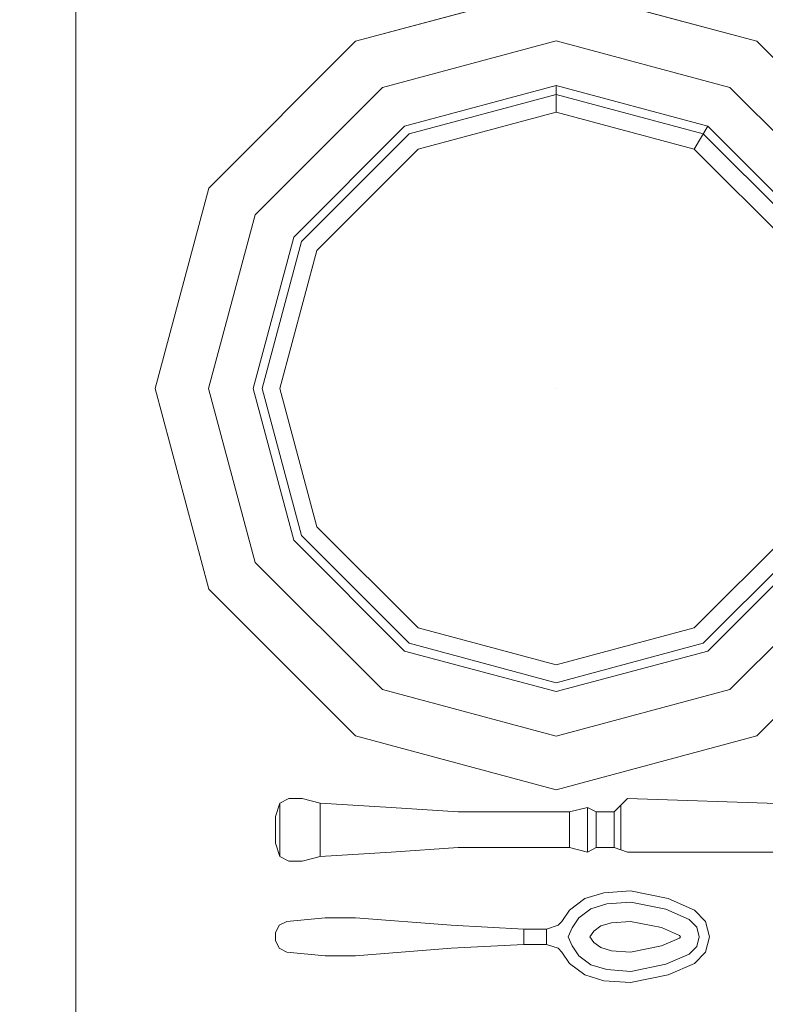
# Model space of a CAD drawing. Units: inches. Extents: x 375 to 1122, y 27 to 1069.
# Tile 116 of 155: x 705.14 to 715.44, y 886.61 to 900.21. Entities that reach past the tile are written whole.
import ezdxf

# ---------------------------------------------------------------- set-up
doc = ezdxf.new("R2010")
doc.units = ezdxf.units.IN
doc.layers.add('A-ANNO-DIMS', color=2, linetype='Continuous', lineweight=18)
doc.layers.add('Furniture', color=30, linetype='Continuous', lineweight=18)
doc.styles.get("Standard").update_dxf_attribs({"font": 'arial.ttf'})
doc.dimstyles.new('ISO-25', dxfattribs={"dimtxt": 12, "dimasz": 2.5, "dimexe": 1.5, "dimexo": 1.5, "dimtad": 1, "dimdec": 1, "dimlunit": 3, "dimtxsty": 'Standard', "dimblk": 'ARCHTICK', "dimcen": 2.5, "dimadec": 0, "dimazin": 0, "dimtfac": 1, "dimtdec": 1, "dimtmove": 0, "dimatfit": 3, "dimfxl": 1.5, "dimfxlon": 1, "dimarcsym": 0})

# ---------------------------------------------------------------- blocks, each defined once
blk = doc.blocks.new('A$C403C54AD')
blk.add_line((0.83575, 0.52421, -0.0006), (1.99923, 0.52421, -0.0006))
at = {"linetype": 'ByBlock'}
for points, invisible_edges in [([(1.01094, 0.81008, -0.00874), (1.02018, 0.79408, -0.00874), (0.97623, 0.75014, -0.00874), (0.96024, 0.75938, -0.00874)], 5), ([(1.02787, 0.78075, -0.02259), (1.01094, 0.81008, -0.01335), (0.96024, 0.75938, -0.01335), (0.98956, 0.74244, -0.02259)], 5), ([(1.17085, 0.74244, -0.02259), (1.20017, 0.75938, -0.01335), (1.14947, 0.81008, -0.01335), (1.13254, 0.78075, -0.02259)], 5), ([(1.20017, 0.75938, -0.00874), (1.18418, 0.75014, -0.00874), (1.14023, 0.79408, -0.00874), (1.14947, 0.81008, -0.00874)], 5), ([(1.02018, 0.79408, -0.00874), (1.02941, 0.77809, -0.01489), (0.99223, 0.74091, -0.01489), (0.97623, 0.75014, -0.00874)], 5), ([(1.18418, 0.75014, -0.00874), (1.16818, 0.74091, -0.01489), (1.131, 0.77809, -0.01489), (1.14023, 0.79408, -0.00874)], 5), ([(1.0802, 0.7917, -0.01489), (1.0802, 0.69011, -0.01489), (1.0802, 0.69011, -0.01489), (1.02941, 0.77809, -0.01489)], 5), ([(1.131, 0.77809, -0.01489), (1.0802, 0.69011, -0.01489), (1.0802, 0.69011, -0.01489), (1.0802, 0.7917, -0.01489)], 5), ([(1.03249, 0.77276, -0.03183), (1.02787, 0.78075, -0.02259), (0.98956, 0.74244, -0.02259), (0.99756, 0.73783, -0.03183)], 1), ([(1.16285, 0.73783, -0.03183), (1.17085, 0.74244, -0.02259), (1.13254, 0.78075, -0.02259), (1.12792, 0.77276, -0.03183)], 5), ([(1.02941, 0.77809, -0.01489), (1.0802, 0.69011, -0.01489), (1.0802, 0.69011, -0.01489), (0.99223, 0.74091, -0.01489)], 5), ([(1.16818, 0.74091, -0.01489), (1.0802, 0.69011, -0.01489), (1.0802, 0.69011, -0.01489), (1.131, 0.77809, -0.01489)], 5), ([(0.96024, 0.75938, -0.00874), (0.97623, 0.75014, -0.00874), (0.96015, 0.69011, -0.00874), (0.94168, 0.69011, -0.00874)], 5), ([(0.98956, 0.74244, -0.02259), (0.96024, 0.75938, -0.01335), (0.94168, 0.69011, -0.01335), (0.97554, 0.69011, -0.02259)], 5), ([(1.18487, 0.69011, -0.02259), (1.21873, 0.69011, -0.01335), (1.20017, 0.75938, -0.01335), (1.17085, 0.74244, -0.02259)], 5), ([(1.21873, 0.69011, -0.00874), (1.20026, 0.69011, -0.00874), (1.18418, 0.75014, -0.00874), (1.20017, 0.75938, -0.00874)], 5), ([(0.97623, 0.75014, -0.00874), (0.99223, 0.74091, -0.01489), (0.97862, 0.69011, -0.01489), (0.96015, 0.69011, -0.00874)], 5), ([(1.20026, 0.69011, -0.00874), (1.18179, 0.69011, -0.01489), (1.16818, 0.74091, -0.01489), (1.18418, 0.75014, -0.00874)], 5), ([(1.17563, 0.69011, -0.03183), (1.18487, 0.69011, -0.02259), (1.17085, 0.74244, -0.02259), (1.16285, 0.73783, -0.03183)], 5), ([(0.99223, 0.74091, -0.01489), (1.0802, 0.69011, -0.01489), (1.0802, 0.69011, -0.01489), (0.97862, 0.69011, -0.01489)], 5), ([(1.18179, 0.69011, -0.01489), (1.0802, 0.69011, -0.01489), (1.0802, 0.69011, -0.01489), (1.16818, 0.74091, -0.01489)], 5), ([(0.94168, 0.69011, -0.00874), (0.96015, 0.69011, -0.00874), (0.97623, 0.63008, -0.00874), (0.96024, 0.62085, -0.00874)], 5), ([(0.97554, 0.69011, -0.02259), (0.94168, 0.69011, -0.01335), (0.96024, 0.62085, -0.01335), (0.98956, 0.63778, -0.02259)], 5), ([(0.96015, 0.69011, -0.00874), (0.97862, 0.69011, -0.01489), (0.99223, 0.63932, -0.01489), (0.97623, 0.63008, -0.00874)], 5), ([(0.98477, 0.69011, -0.03183), (0.97554, 0.69011, -0.02259), (0.98956, 0.63778, -0.02259), (0.99756, 0.6424, -0.03183)], 4), ([(0.97862, 0.69011, -0.01489), (1.0802, 0.69011, -0.01489), (1.0802, 0.69011, -0.01489), (0.99223, 0.63932, -0.01489)], 5), ([(0.99223, 0.63932, -0.01489), (1.0802, 0.69011, -0.01489), (1.0802, 0.69011, -0.01489), (1.02941, 0.60214, -0.01489)], 5), ([(1.02941, 0.60214, -0.01489), (1.0802, 0.69011, -0.01489), (1.0802, 0.69011, -0.01489), (1.0802, 0.58853, -0.01489)], 5), ([(1.0802, 0.58853, -0.01489), (1.0802, 0.69011, -0.01489), (1.0802, 0.69011, -0.01489), (1.131, 0.60214, -0.01489)], 5), ([(1.131, 0.60214, -0.01489), (1.0802, 0.69011, -0.01489), (1.0802, 0.69011, -0.01489), (1.16818, 0.63932, -0.01489)], 5), ([(1.16818, 0.63932, -0.01489), (1.0802, 0.69011, -0.01489), (1.0802, 0.69011, -0.01489), (1.18179, 0.69011, -0.01489)], 5), ([(1.16285, 0.6424, -0.03183), (1.17085, 0.63778, -0.02259), (1.18487, 0.69011, -0.02259), (1.17563, 0.69011, -0.03183)], 5), ([(1.18418, 0.63008, -0.00874), (1.16818, 0.63932, -0.01489), (1.18179, 0.69011, -0.01489), (1.20026, 0.69011, -0.00874)], 5), ([(1.17085, 0.63778, -0.02259), (1.20017, 0.62085, -0.01335), (1.21873, 0.69011, -0.01335), (1.18487, 0.69011, -0.02259)], 5), ([(1.20017, 0.62085, -0.00874), (1.18418, 0.63008, -0.00874), (1.20026, 0.69011, -0.00874), (1.21873, 0.69011, -0.00874)], 5), ([(0.97623, 0.63008, -0.00874), (0.99223, 0.63932, -0.01489), (1.02941, 0.60214, -0.01489), (1.02018, 0.58614, -0.00874)], 5), ([(0.99756, 0.6424, -0.03183), (0.98956, 0.63778, -0.02259), (1.02787, 0.59947, -0.02259), (1.03249, 0.60747, -0.03183)], 5), ([(1.12792, 0.60747, -0.03183), (1.13254, 0.59947, -0.02259), (1.17085, 0.63778, -0.02259), (1.16285, 0.6424, -0.03183)], 5), ([(1.14023, 0.58614, -0.00874), (1.131, 0.60214, -0.01489), (1.16818, 0.63932, -0.01489), (1.18418, 0.63008, -0.00874)], 5), ([(0.98956, 0.63778, -0.02259), (0.96024, 0.62085, -0.01335), (1.01094, 0.57014, -0.01335), (1.02787, 0.59947, -0.02259)], 5), ([(1.13254, 0.59947, -0.02259), (1.14947, 0.57014, -0.01335), (1.20017, 0.62085, -0.01335), (1.17085, 0.63778, -0.02259)], 5), ([(0.96024, 0.62085, -0.00874), (0.97623, 0.63008, -0.00874), (1.02018, 0.58614, -0.00874), (1.01094, 0.57014, -0.00874)], 5), ([(1.14947, 0.57014, -0.00874), (1.14023, 0.58614, -0.00874), (1.18418, 0.63008, -0.00874), (1.20017, 0.62085, -0.00874)], 5), ([(1.03249, 0.60747, -0.03183), (1.02787, 0.59947, -0.02259), (1.0802, 0.58545, -0.02259), (1.0802, 0.59468, -0.03183)], 5), ([(1.0802, 0.59468, -0.03183), (1.0802, 0.58545, -0.02259), (1.13254, 0.59947, -0.02259), (1.12792, 0.60747, -0.03183)], 5), ([(1.02018, 0.58614, -0.00874), (1.02941, 0.60214, -0.01489), (1.0802, 0.58853, -0.01489), (1.0802, 0.57006, -0.00874)], 5), ([(1.0802, 0.57006, -0.00874), (1.0802, 0.58853, -0.01489), (1.131, 0.60214, -0.01489), (1.14023, 0.58614, -0.00874)], 5), ([(1.02787, 0.59947, -0.02259), (1.01094, 0.57014, -0.01335), (1.0802, 0.55159, -0.01335), (1.0802, 0.58545, -0.02259)], 5), ([(1.0802, 0.58545, -0.02259), (1.0802, 0.55159, -0.01335), (1.14947, 0.57014, -0.01335), (1.13254, 0.59947, -0.02259)], 5), ([(1.01094, 0.57014, -0.00874), (1.02018, 0.58614, -0.00874), (1.0802, 0.57006, -0.00874), (1.0802, 0.55159, -0.00874)], 5), ([(1.0802, 0.55159, -0.00874), (1.0802, 0.57006, -0.00874), (1.14023, 0.58614, -0.00874), (1.14947, 0.57014, -0.00874)], 5)]:
    blk.add_3dface(points, dxfattribs=dict(at, invisible_edges=invisible_edges))
for points in [[(1.01094, 0.81008, -0.01335), (1.01094, 0.81008, -0.00874), (0.96024, 0.75938, -0.00874), (0.96024, 0.75938, -0.01335)], [(1.20017, 0.75938, -0.01335), (1.20017, 0.75938, -0.00874), (1.14947, 0.81008, -0.00874), (1.14947, 0.81008, -0.01335)], [(0.96024, 0.75938, -0.01335), (0.96024, 0.75938, -0.00874), (0.94168, 0.69011, -0.00874), (0.94168, 0.69011, -0.01335)], [(1.21873, 0.69011, -0.01335), (1.21873, 0.69011, -0.00874), (1.20017, 0.75938, -0.00874), (1.20017, 0.75938, -0.01335)], [(0.99756, 0.73783, -0.03183), (0.98956, 0.74244, -0.02259), (0.97554, 0.69011, -0.02259), (0.98477, 0.69011, -0.03183)], [(0.94168, 0.69011, -0.01335), (0.94168, 0.69011, -0.00874), (0.96024, 0.62085, -0.00874), (0.96024, 0.62085, -0.01335)], [(1.20017, 0.62085, -0.01335), (1.20017, 0.62085, -0.00874), (1.21873, 0.69011, -0.00874), (1.21873, 0.69011, -0.01335)], [(0.96024, 0.62085, -0.01335), (0.96024, 0.62085, -0.00874), (1.01094, 0.57014, -0.00874), (1.01094, 0.57014, -0.01335)], [(1.14947, 0.57014, -0.01335), (1.14947, 0.57014, -0.00874), (1.20017, 0.62085, -0.00874), (1.20017, 0.62085, -0.01335)], [(1.01094, 0.57014, -0.01335), (1.01094, 0.57014, -0.00874), (1.0802, 0.55159, -0.00874), (1.0802, 0.55159, -0.01335)], [(1.0802, 0.55159, -0.01335), (1.0802, 0.55159, -0.00874), (1.14947, 0.57014, -0.00874), (1.14947, 0.57014, -0.01335)]]:
    blk.add_3dface(points, dxfattribs=at)
for points, invisible_edges in [([(1.24028, 0.77323, -0.0249), (1.22489, 0.81171, -0.0249), (1.22181, 0.71474, -0.0249), (1.24028, 0.71474, -0.0249)], 5), ([(1.24028, 0.77323, -0.02644), (1.22489, 0.81171, -0.02644), (1.22181, 0.71474, -0.02644), (1.24028, 0.71474, -0.02644)], 5), ([(1.22489, 0.81171, -0.02644), (1.22489, 0.81171, -0.0249), (1.22181, 0.71474, -0.0249), (1.22181, 0.71474, -0.02644)], 5), ([(1.24028, 0.71474, -0.0249), (1.24028, 0.71474, -0.02644), (1.24028, 0.77323, -0.02644), (1.24028, 0.77323, -0.0249)], 5), ([(1.26354, 0.73605, -0.02421), (1.26029, 0.73789, -0.02157), (1.26425, 0.74173, -0.02048), (1.26622, 0.73867, -0.02365)], 5), ([(1.26354, 0.73605, -0.02289), (1.26029, 0.73789, -0.02025), (1.26425, 0.74173, -0.01916), (1.26622, 0.73867, -0.02233)], 5), ([(1.26425, 0.74173, -0.02048), (1.26622, 0.73867, -0.02365), (1.26953, 0.73948, -0.02346), (1.26953, 0.74304, -0.02029)], 5), ([(1.26425, 0.74173, -0.01916), (1.26622, 0.73867, -0.02233), (1.26953, 0.73948, -0.02215), (1.26953, 0.74304, -0.01897)], 5), ([(1.2748, 0.74173, -0.02048), (1.27283, 0.73867, -0.02365), (1.26953, 0.73948, -0.02346), (1.26953, 0.74304, -0.02029)], 5), ([(1.2748, 0.74173, -0.01916), (1.27283, 0.73867, -0.02233), (1.26953, 0.73948, -0.02215), (1.26953, 0.74304, -0.01897)], 5), ([(1.27551, 0.73605, -0.02421), (1.27876, 0.73789, -0.02157), (1.2748, 0.74173, -0.02048), (1.27283, 0.73867, -0.02365)], 5), ([(1.27551, 0.73605, -0.02289), (1.27876, 0.73789, -0.02025), (1.2748, 0.74173, -0.01916), (1.27283, 0.73867, -0.02233)], 5), ([(1.25633, 0.72882, -0.0234), (1.26003, 0.72802, -0.02592), (1.26354, 0.73605, -0.02421), (1.26029, 0.73789, -0.02157)], 5), ([(1.25633, 0.72882, -0.02208), (1.26003, 0.72802, -0.0246), (1.26354, 0.73605, -0.02289), (1.26029, 0.73789, -0.02025)], 5), ([(1.26909, 0.73267, -0.02578), (1.26622, 0.73867, -0.02233), (1.26354, 0.73605, -0.02289), (1.26909, 0.73267, -0.02578)], 5), ([(1.26909, 0.73267, -0.0271), (1.26622, 0.73867, -0.02365), (1.26354, 0.73605, -0.02421), (1.26909, 0.73267, -0.0271)], 5), ([(1.26953, 0.73948, -0.02215), (1.26953, 0.73309, -0.02564), (1.26909, 0.73267, -0.02578), (1.26622, 0.73867, -0.02233)], 5), ([(1.26953, 0.73948, -0.02346), (1.26953, 0.73309, -0.02696), (1.26909, 0.73267, -0.0271), (1.26622, 0.73867, -0.02365)], 5), ([(1.26953, 0.73948, -0.02215), (1.26953, 0.73309, -0.02564), (1.26996, 0.73267, -0.02578), (1.27283, 0.73867, -0.02233)], 5), ([(1.26953, 0.73948, -0.02346), (1.26953, 0.73309, -0.02696), (1.26996, 0.73267, -0.0271), (1.27283, 0.73867, -0.02365)], 5), ([(1.26996, 0.73267, -0.02578), (1.27283, 0.73867, -0.02233), (1.27551, 0.73605, -0.02289), (1.26996, 0.73267, -0.02578)], 5), ([(1.26996, 0.73267, -0.0271), (1.27283, 0.73867, -0.02365), (1.27551, 0.73605, -0.02421), (1.26996, 0.73267, -0.0271)], 5), ([(1.28272, 0.72882, -0.0234), (1.27902, 0.72802, -0.02592), (1.27551, 0.73605, -0.02421), (1.27876, 0.73789, -0.02157)], 5), ([(1.28272, 0.72882, -0.02208), (1.27902, 0.72802, -0.0246), (1.27551, 0.73605, -0.02289), (1.27876, 0.73789, -0.02025)], 5), ([(1.26354, 0.73605, -0.02421), (1.26909, 0.73267, -0.0271), (1.26635, 0.72644, -0.02873), (1.26003, 0.72802, -0.02592)], 5), ([(1.26354, 0.73605, -0.02289), (1.26909, 0.73267, -0.02578), (1.26635, 0.72644, -0.02741), (1.26003, 0.72802, -0.0246)], 5), ([(1.27551, 0.73605, -0.02421), (1.26996, 0.73267, -0.0271), (1.2727, 0.72644, -0.02873), (1.27902, 0.72802, -0.02592)], 5), ([(1.27551, 0.73605, -0.02289), (1.26996, 0.73267, -0.02578), (1.2727, 0.72644, -0.02741), (1.27902, 0.72802, -0.0246)], 5), ([(1.26909, 0.73267, -0.0271), (1.26996, 0.73267, -0.0271), (1.2727, 0.72644, -0.02873), (1.26635, 0.72644, -0.02873)], 5), ([(1.26909, 0.73267, -0.02578), (1.26996, 0.73267, -0.02578), (1.2727, 0.72644, -0.02741), (1.26635, 0.72644, -0.02741)], 5), ([(1.26953, 0.73309, -0.02564), (1.26996, 0.73267, -0.02578), (1.26909, 0.73267, -0.02578), (1.26953, 0.73309, -0.02564)], 2), ([(1.26953, 0.73309, -0.02696), (1.26996, 0.73267, -0.0271), (1.26909, 0.73267, -0.0271), (1.26953, 0.73309, -0.02696)], 2), ([(1.25757, 0.71589, -0.0279), (1.25369, 0.71579, -0.02544), (1.25633, 0.72882, -0.0234), (1.26003, 0.72802, -0.02592)], 5), ([(1.25757, 0.71589, -0.02658), (1.25369, 0.71579, -0.02412), (1.25633, 0.72882, -0.02208), (1.26003, 0.72802, -0.0246)], 5), ([(1.26635, 0.72644, -0.02741), (1.26003, 0.72802, -0.0246), (1.25757, 0.71589, -0.02658), (1.2642, 0.71583, -0.02912)], 5), ([(1.26635, 0.72644, -0.02873), (1.26003, 0.72802, -0.02592), (1.25757, 0.71589, -0.0279), (1.2642, 0.71583, -0.03044)], 5), ([(1.2727, 0.72644, -0.02741), (1.27902, 0.72802, -0.0246), (1.28148, 0.71589, -0.02658), (1.27485, 0.71583, -0.02912)], 5), ([(1.2727, 0.72644, -0.02873), (1.27902, 0.72802, -0.02592), (1.28148, 0.71589, -0.0279), (1.27485, 0.71583, -0.03044)], 5), ([(1.28148, 0.71589, -0.0279), (1.28536, 0.71579, -0.02544), (1.28272, 0.72882, -0.0234), (1.27902, 0.72802, -0.02592)], 5), ([(1.28148, 0.71589, -0.02658), (1.28536, 0.71579, -0.02412), (1.28272, 0.72882, -0.02208), (1.27902, 0.72802, -0.0246)], 5), ([(1.2727, 0.72644, -0.02741), (1.26635, 0.72644, -0.02741), (1.2642, 0.71583, -0.02912), (1.27485, 0.71583, -0.02912)], 5), ([(1.2727, 0.72644, -0.02873), (1.26635, 0.72644, -0.02873), (1.2642, 0.71583, -0.03044), (1.27485, 0.71583, -0.03044)], 5), ([(1.22181, 0.71474, -0.0249), (1.24028, 0.71474, -0.0249), (1.23951, 0.71243, -0.02413), (1.22412, 0.71243, -0.02413)], 1), ([(1.22181, 0.71474, -0.02644), (1.24028, 0.71474, -0.02644), (1.23951, 0.71243, -0.02721), (1.22412, 0.71243, -0.02721)], 1), ([(1.22181, 0.71474, -0.02644), (1.22181, 0.71474, -0.0249), (1.22412, 0.71243, -0.02413), (1.22412, 0.71243, -0.02721)], 5), ([(1.23951, 0.71243, -0.02721), (1.23951, 0.71243, -0.02413), (1.24028, 0.71474, -0.0249), (1.24028, 0.71474, -0.02644)], 5), ([(1.25435, 0.70658, -0.02499), (1.25817, 0.70765, -0.02747), (1.25757, 0.71589, -0.02658), (1.25369, 0.71579, -0.02412)], 5), ([(1.25435, 0.70658, -0.02631), (1.25817, 0.70765, -0.02879), (1.25757, 0.71589, -0.0279), (1.25369, 0.71579, -0.02544)], 5), ([(1.25757, 0.71589, -0.0279), (1.2642, 0.71583, -0.03044), (1.26468, 0.70922, -0.03139), (1.25817, 0.70765, -0.02879)], 5), ([(1.25757, 0.71589, -0.02658), (1.2642, 0.71583, -0.02912), (1.26468, 0.70922, -0.03007), (1.25817, 0.70765, -0.02747)], 5), ([(1.2642, 0.71583, -0.03044), (1.27485, 0.71583, -0.03044), (1.27437, 0.70922, -0.03139), (1.26468, 0.70922, -0.03139)], 5), ([(1.2642, 0.71583, -0.02912), (1.27485, 0.71583, -0.02912), (1.27437, 0.70922, -0.03007), (1.26468, 0.70922, -0.03007)], 5), ([(1.28148, 0.71589, -0.0279), (1.27485, 0.71583, -0.03044), (1.27437, 0.70922, -0.03139), (1.28088, 0.70765, -0.02879)], 5), ([(1.28148, 0.71589, -0.02658), (1.27485, 0.71583, -0.02912), (1.27437, 0.70922, -0.03007), (1.28088, 0.70765, -0.02747)], 5), ([(1.2847, 0.70658, -0.02499), (1.28088, 0.70765, -0.02747), (1.28148, 0.71589, -0.02658), (1.28536, 0.71579, -0.02412)], 5), ([(1.2847, 0.70658, -0.02631), (1.28088, 0.70765, -0.02879), (1.28148, 0.71589, -0.0279), (1.28536, 0.71579, -0.02544)], 5), ([(1.22412, 0.71243, -0.02413), (1.22412, 0.71243, -0.02721), (1.22643, 0.71012, -0.03029), (1.22643, 0.71012, -0.02105)], 5), ([(1.23874, 0.71012, -0.02105), (1.23874, 0.71012, -0.03029), (1.23951, 0.71243, -0.02721), (1.23951, 0.71243, -0.02413)], 5), ([(1.22643, 0.71012, -0.03029), (1.22643, 0.71012, -0.02105), (1.22643, 0.70396, -0.02105), (1.22643, 0.70396, -0.03029)], 1), ([(1.23874, 0.70396, -0.03029), (1.23874, 0.70396, -0.02105), (1.23874, 0.71012, -0.02105), (1.23874, 0.71012, -0.03029)], 4), ([(1.25983, 0.70213, -0.02798), (1.25633, 0.69998, -0.02539), (1.25435, 0.70658, -0.02499), (1.25817, 0.70765, -0.02747)], 5), ([(1.25983, 0.70213, -0.0293), (1.25633, 0.69998, -0.02671), (1.25435, 0.70658, -0.02631), (1.25817, 0.70765, -0.02879)], 5), ([(1.26468, 0.70922, -0.03007), (1.25817, 0.70765, -0.02747), (1.25983, 0.70213, -0.02798), (1.26579, 0.7055, -0.0303)], 5), ([(1.27437, 0.70922, -0.03139), (1.26468, 0.70922, -0.03139), (1.26579, 0.7055, -0.03162), (1.27326, 0.7055, -0.03162)], 5), ([(1.27437, 0.70922, -0.03007), (1.26468, 0.70922, -0.03007), (1.26579, 0.7055, -0.0303), (1.27326, 0.7055, -0.0303)], 5), ([(1.27437, 0.70922, -0.03139), (1.28088, 0.70765, -0.02879), (1.27922, 0.70213, -0.0293), (1.27326, 0.7055, -0.03162)], 5), ([(1.27437, 0.70922, -0.03007), (1.28088, 0.70765, -0.02747), (1.27922, 0.70213, -0.02798), (1.27326, 0.7055, -0.0303)], 5), ([(1.27922, 0.70213, -0.02798), (1.28272, 0.69998, -0.02539), (1.2847, 0.70658, -0.02499), (1.28088, 0.70765, -0.02747)], 5), ([(1.27922, 0.70213, -0.0293), (1.28272, 0.69998, -0.02671), (1.2847, 0.70658, -0.02631), (1.28088, 0.70765, -0.02879)], 5), ([(1.25983, 0.70213, -0.0293), (1.26579, 0.7055, -0.03162), (1.26756, 0.70313, -0.03172), (1.26298, 0.69791, -0.02947)], 5), ([(1.25983, 0.70213, -0.02798), (1.26579, 0.7055, -0.0303), (1.26756, 0.70313, -0.0304), (1.26298, 0.69791, -0.02815)], 5), ([(1.26579, 0.7055, -0.03162), (1.27326, 0.7055, -0.03162), (1.27149, 0.70313, -0.03172), (1.26756, 0.70313, -0.03172)], 5), ([(1.26579, 0.7055, -0.0303), (1.27326, 0.7055, -0.0303), (1.27149, 0.70313, -0.0304), (1.26756, 0.70313, -0.0304)], 5), ([(1.27922, 0.70213, -0.0293), (1.27326, 0.7055, -0.03162), (1.27149, 0.70313, -0.03172), (1.27607, 0.69791, -0.02947)], 5), ([(1.27922, 0.70213, -0.02798), (1.27326, 0.7055, -0.0303), (1.27149, 0.70313, -0.0304), (1.27607, 0.69791, -0.02815)], 5), ([(1.26029, 0.69472, -0.02719), (1.26298, 0.69791, -0.02947), (1.25983, 0.70213, -0.0293), (1.25633, 0.69998, -0.02671)], 5), ([(1.26029, 0.69472, -0.02588), (1.26298, 0.69791, -0.02815), (1.25983, 0.70213, -0.02798), (1.25633, 0.69998, -0.02539)], 5), ([(1.26756, 0.70313, -0.03172), (1.26298, 0.69791, -0.02947), (1.26639, 0.69562, -0.02948), (1.26953, 0.70178, -0.03152)], 5), ([(1.26756, 0.70313, -0.0304), (1.26298, 0.69791, -0.02815), (1.26639, 0.69562, -0.02816), (1.26953, 0.70178, -0.0302)], 5), ([(1.26639, 0.69562, -0.02948), (1.26953, 0.70178, -0.03152), (1.26953, 0.70178, -0.03152), (1.26953, 0.69426, -0.0293)], 5), ([(1.26639, 0.69562, -0.02816), (1.26953, 0.70178, -0.0302), (1.26953, 0.70178, -0.0302), (1.26953, 0.69426, -0.02798)], 5), ([(1.27149, 0.70313, -0.03172), (1.26756, 0.70313, -0.03172), (1.26953, 0.70178, -0.03152)], 1), ([(1.27149, 0.70313, -0.0304), (1.26756, 0.70313, -0.0304), (1.26953, 0.70178, -0.0302)], 1), ([(1.27149, 0.70313, -0.03172), (1.27607, 0.69791, -0.02947), (1.27266, 0.69562, -0.02948), (1.26953, 0.70178, -0.03152)], 5), ([(1.27149, 0.70313, -0.0304), (1.27607, 0.69791, -0.02815), (1.27266, 0.69562, -0.02816), (1.26953, 0.70178, -0.0302)], 5), ([(1.27266, 0.69562, -0.02948), (1.26953, 0.70178, -0.03152), (1.26953, 0.70178, -0.03152), (1.26953, 0.69426, -0.0293)], 5), ([(1.27266, 0.69562, -0.02816), (1.26953, 0.70178, -0.0302), (1.26953, 0.70178, -0.0302), (1.26953, 0.69426, -0.02798)], 5), ([(1.27876, 0.69472, -0.02719), (1.27607, 0.69791, -0.02947), (1.27922, 0.70213, -0.0293), (1.28272, 0.69998, -0.02671)], 5), ([(1.27876, 0.69472, -0.02588), (1.27607, 0.69791, -0.02815), (1.27922, 0.70213, -0.02798), (1.28272, 0.69998, -0.02539)], 5), ([(1.26639, 0.69562, -0.02816), (1.26425, 0.6921, -0.02625), (1.26029, 0.69472, -0.02588), (1.26298, 0.69791, -0.02815)], 5), ([(1.27266, 0.69562, -0.02948), (1.2748, 0.6921, -0.0284), (1.27876, 0.69472, -0.02719), (1.27607, 0.69791, -0.02947)], 5), ([(1.27266, 0.69562, -0.02816), (1.2748, 0.6921, -0.02625), (1.27876, 0.69472, -0.02588), (1.27607, 0.69791, -0.02815)], 5), ([(1.22643, 0.69473, -0.02105), (1.23874, 0.69473, -0.02105), (1.23874, 0.65625, -0.01951), (1.22643, 0.65625, -0.01951)], 4), ([(1.22643, 0.69473, -0.03029), (1.23874, 0.69473, -0.03029), (1.23874, 0.65625, -0.03183), (1.22643, 0.65625, -0.03183)], 4), ([(1.26425, 0.6921, -0.0284), (1.26953, 0.6921, -0.0284), (1.26953, 0.69426, -0.0293), (1.26639, 0.69562, -0.02948)], 11), ([(1.26425, 0.6921, -0.02625), (1.26953, 0.6921, -0.02625), (1.26953, 0.69426, -0.02798), (1.26639, 0.69562, -0.02816)], 11), ([(1.2748, 0.6921, -0.0284), (1.26953, 0.6921, -0.0284), (1.26953, 0.69426, -0.0293), (1.27266, 0.69562, -0.02948)], 11), ([(1.2748, 0.6921, -0.02625), (1.26953, 0.6921, -0.02625), (1.26953, 0.69426, -0.02798), (1.27266, 0.69562, -0.02816)], 11), ([(1.26557, 0.69077, -0.02551), (1.27348, 0.69077, -0.02551), (1.2748, 0.6921, -0.02625), (1.26425, 0.6921, -0.02625)], 5), ([(1.26557, 0.69077, -0.0276), (1.27348, 0.69077, -0.0276), (1.2748, 0.6921, -0.0284), (1.26425, 0.6921, -0.0284)], 5), ([(1.26557, 0.69077, -0.02551), (1.26557, 0.69077, -0.0276), (1.26425, 0.6921, -0.0284), (1.26425, 0.6921, -0.02625)], 1), ([(1.27216, 0.68681, -0.02366), (1.26689, 0.68681, -0.02366), (1.26557, 0.69077, -0.02551), (1.27348, 0.69077, -0.02551)], 4), ([(1.26689, 0.68681, -0.02588), (1.26689, 0.68681, -0.02366), (1.26557, 0.69077, -0.02551), (1.26557, 0.69077, -0.0276)], 5), ([(1.27216, 0.68681, -0.02588), (1.26689, 0.68681, -0.02588), (1.26557, 0.69077, -0.0276), (1.27348, 0.69077, -0.0276)], 4), ([(1.27216, 0.68681, -0.02366), (1.27216, 0.68681, -0.02588), (1.27348, 0.69077, -0.0276), (1.27348, 0.69077, -0.02551)], 5), ([(1.27348, 0.69077, -0.0276), (1.27348, 0.69077, -0.02551), (1.2748, 0.6921, -0.02625), (1.2748, 0.6921, -0.0284)], 1), ([(1.26689, 0.68681, -0.02588), (1.26689, 0.68681, -0.02366), (1.26689, 0.6789, -0.02303), (1.26689, 0.6789, -0.02525)], 5), ([(1.27216, 0.6789, -0.02525), (1.27216, 0.6789, -0.02303), (1.27216, 0.68681, -0.02366), (1.27216, 0.68681, -0.02588)], 5), ([(1.27348, 0.65383, -0.02553), (1.26557, 0.65383, -0.02553), (1.26689, 0.6789, -0.02303), (1.27216, 0.6789, -0.02303)], 1), ([(1.26689, 0.6789, -0.02303), (1.26689, 0.6789, -0.02525), (1.26557, 0.65383, -0.02816), (1.26557, 0.65383, -0.02553)], 5), ([(1.27348, 0.65383, -0.02816), (1.26557, 0.65383, -0.02816), (1.26689, 0.6789, -0.02525), (1.27216, 0.6789, -0.02525)], 1), ([(1.27348, 0.65383, -0.02553), (1.27348, 0.65383, -0.02816), (1.27216, 0.6789, -0.02525), (1.27216, 0.6789, -0.02303)], 5), ([(1.23874, 0.65625, -0.01951), (1.22643, 0.65625, -0.01951), (1.22489, 0.63316, -0.01951), (1.24028, 0.63316, -0.01951)], 5), ([(1.23874, 0.65625, -0.03183), (1.22643, 0.65625, -0.03183), (1.22489, 0.63316, -0.03183), (1.24028, 0.63316, -0.03183)], 5), ([(1.26293, 0.62085, -0.03154), (1.27612, 0.62085, -0.03154), (1.27348, 0.65383, -0.02816), (1.26557, 0.65383, -0.02816)], 5), ([(1.26557, 0.65383, -0.02816), (1.26557, 0.65383, -0.02553), (1.26293, 0.62085, -0.02757), (1.26293, 0.62085, -0.03154)], 1), ([(1.26293, 0.62085, -0.02757), (1.27612, 0.62085, -0.02757), (1.27348, 0.65383, -0.02553), (1.26557, 0.65383, -0.02553)], 5), ([(1.27612, 0.62085, -0.03154), (1.27612, 0.62085, -0.02757), (1.27348, 0.65383, -0.02553), (1.27348, 0.65383, -0.02816)], 4), ([(1.22489, 0.63316, -0.01951), (1.24028, 0.63316, -0.01951), (1.24182, 0.60854, -0.02105), (1.22335, 0.60854, -0.02105)], 1), ([(1.22489, 0.63316, -0.03183), (1.24028, 0.63316, -0.03183), (1.24182, 0.60854, -0.03029), (1.22335, 0.60854, -0.03029)], 1), ([(1.27612, 0.61029, -0.02785), (1.26293, 0.61029, -0.02785), (1.26293, 0.62085, -0.02757), (1.27612, 0.62085, -0.02757)], 5), ([(1.27612, 0.61029, -0.03182), (1.26293, 0.61029, -0.03182), (1.26293, 0.62085, -0.03154), (1.27612, 0.62085, -0.03154)], 5), ([(1.26425, 0.5971, -0.02782), (1.2748, 0.5971, -0.02782), (1.27612, 0.61029, -0.02785), (1.26293, 0.61029, -0.02785)], 5), ([(1.26425, 0.5971, -0.03179), (1.2748, 0.5971, -0.03179), (1.27612, 0.61029, -0.03182), (1.26293, 0.61029, -0.03182)], 5), ([(1.24182, 0.60854, -0.02105), (1.22335, 0.60854, -0.02105), (1.22181, 0.60238, -0.01951), (1.24336, 0.60238, -0.01951)], 4), ([(1.24182, 0.60854, -0.03029), (1.22335, 0.60854, -0.03029), (1.22181, 0.60238, -0.03183), (1.24336, 0.60238, -0.03183)], 4), ([(1.22181, 0.60238, -0.01951), (1.24336, 0.60238, -0.01951), (1.24336, 0.59776, -0.02105), (1.22181, 0.59776, -0.02105)], 5), ([(1.22181, 0.60238, -0.03183), (1.24336, 0.60238, -0.03183), (1.24336, 0.59776, -0.03029), (1.22181, 0.59776, -0.03029)], 5), ([(1.24336, 0.59776, -0.02105), (1.22181, 0.59776, -0.02105), (1.22335, 0.59468, -0.02259), (1.24182, 0.59468, -0.02259)], 1), ([(1.24336, 0.59776, -0.03029), (1.22181, 0.59776, -0.03029), (1.22335, 0.59468, -0.02875), (1.24182, 0.59468, -0.02875)], 1), ([(1.27348, 0.59446, -0.02761), (1.26557, 0.59446, -0.02761), (1.26425, 0.5971, -0.02782), (1.2748, 0.5971, -0.02782)], 5), ([(1.27348, 0.59446, -0.03158), (1.26557, 0.59446, -0.03158), (1.26425, 0.5971, -0.03179), (1.2748, 0.5971, -0.03179)], 5), ([(1.26821, 0.59314, -0.02775), (1.27084, 0.59314, -0.02775), (1.27348, 0.59446, -0.02761), (1.26557, 0.59446, -0.02761)], 4), ([(1.26821, 0.59314, -0.0313), (1.27084, 0.59314, -0.0313), (1.27348, 0.59446, -0.03158), (1.26557, 0.59446, -0.03158)], 4)]:
    blk.add_3dface(points, dxfattribs=dict(invisible_edges=invisible_edges))
for points in [[(1.26425, 0.74173, -0.01916), (1.26425, 0.74173, -0.02048), (1.26029, 0.73789, -0.02157), (1.26029, 0.73789, -0.02025)], [(1.26953, 0.74304, -0.02029), (1.26953, 0.74304, -0.01897), (1.26425, 0.74173, -0.01916), (1.26425, 0.74173, -0.02048)], [(1.2748, 0.74173, -0.01916), (1.2748, 0.74173, -0.02048), (1.26953, 0.74304, -0.02029), (1.26953, 0.74304, -0.01897)], [(1.27876, 0.73789, -0.02157), (1.27876, 0.73789, -0.02025), (1.2748, 0.74173, -0.01916), (1.2748, 0.74173, -0.02048)], [(1.26029, 0.73789, -0.02157), (1.26029, 0.73789, -0.02025), (1.25633, 0.72882, -0.02208), (1.25633, 0.72882, -0.0234)], [(1.28272, 0.72882, -0.02208), (1.28272, 0.72882, -0.0234), (1.27876, 0.73789, -0.02157), (1.27876, 0.73789, -0.02025)], [(1.25633, 0.72882, -0.02208), (1.25633, 0.72882, -0.0234), (1.25369, 0.71579, -0.02544), (1.25369, 0.71579, -0.02412)], [(1.28536, 0.71579, -0.02544), (1.28536, 0.71579, -0.02412), (1.28272, 0.72882, -0.02208), (1.28272, 0.72882, -0.0234)], [(1.25369, 0.71579, -0.02544), (1.25369, 0.71579, -0.02412), (1.25435, 0.70658, -0.02499), (1.25435, 0.70658, -0.02631)], [(1.2847, 0.70658, -0.02499), (1.2847, 0.70658, -0.02631), (1.28536, 0.71579, -0.02544), (1.28536, 0.71579, -0.02412)], [(1.22412, 0.71243, -0.02413), (1.23951, 0.71243, -0.02413), (1.23874, 0.71012, -0.02105), (1.22643, 0.71012, -0.02105)], [(1.22412, 0.71243, -0.02721), (1.23951, 0.71243, -0.02721), (1.23874, 0.71012, -0.03029), (1.22643, 0.71012, -0.03029)], [(1.23874, 0.71012, -0.02105), (1.22643, 0.71012, -0.02105), (1.22643, 0.70396, -0.02105), (1.23874, 0.70396, -0.02105)], [(1.23874, 0.71012, -0.03029), (1.22643, 0.71012, -0.03029), (1.22643, 0.70396, -0.03029), (1.23874, 0.70396, -0.03029)], [(1.22643, 0.70396, -0.02105), (1.23874, 0.70396, -0.02105), (1.24028, 0.70089, -0.01951), (1.22489, 0.70089, -0.01951)], [(1.22643, 0.70396, -0.03029), (1.23874, 0.70396, -0.03029), (1.24028, 0.70089, -0.03183), (1.22489, 0.70089, -0.03183)], [(1.22643, 0.70396, -0.02105), (1.22643, 0.70396, -0.03029), (1.22489, 0.70089, -0.03183), (1.22489, 0.70089, -0.01951)], [(1.24028, 0.70089, -0.01951), (1.24028, 0.70089, -0.03183), (1.23874, 0.70396, -0.03029), (1.23874, 0.70396, -0.02105)], [(1.25435, 0.70658, -0.02631), (1.25435, 0.70658, -0.02499), (1.25633, 0.69998, -0.02539), (1.25633, 0.69998, -0.02671)], [(1.28272, 0.69998, -0.02671), (1.28272, 0.69998, -0.02539), (1.2847, 0.70658, -0.02499), (1.2847, 0.70658, -0.02631)], [(1.24028, 0.70089, -0.01951), (1.22489, 0.70089, -0.01951), (1.22643, 0.69473, -0.02105), (1.23874, 0.69473, -0.02105)], [(1.24028, 0.70089, -0.03183), (1.22489, 0.70089, -0.03183), (1.22643, 0.69473, -0.03029), (1.23874, 0.69473, -0.03029)], [(1.22489, 0.70089, -0.03183), (1.22489, 0.70089, -0.01951), (1.22643, 0.69473, -0.02105), (1.22643, 0.69473, -0.03029)], [(1.23874, 0.69473, -0.03029), (1.23874, 0.69473, -0.02105), (1.24028, 0.70089, -0.01951), (1.24028, 0.70089, -0.03183)], [(1.25633, 0.69998, -0.02539), (1.25633, 0.69998, -0.02671), (1.26029, 0.69472, -0.02719), (1.26029, 0.69472, -0.02588)], [(1.27876, 0.69472, -0.02588), (1.27876, 0.69472, -0.02719), (1.28272, 0.69998, -0.02671), (1.28272, 0.69998, -0.02539)], [(1.22643, 0.69473, -0.02105), (1.22643, 0.69473, -0.03029), (1.22643, 0.65625, -0.03183), (1.22643, 0.65625, -0.01951)], [(1.23874, 0.65625, -0.01951), (1.23874, 0.65625, -0.03183), (1.23874, 0.69473, -0.03029), (1.23874, 0.69473, -0.02105)], [(1.26029, 0.69472, -0.02719), (1.26029, 0.69472, -0.02588), (1.26425, 0.6921, -0.02625), (1.26425, 0.6921, -0.0284)], [(1.2748, 0.6921, -0.0284), (1.2748, 0.6921, -0.02625), (1.27876, 0.69472, -0.02588), (1.27876, 0.69472, -0.02719)], [(1.26689, 0.6789, -0.02525), (1.27216, 0.6789, -0.02525), (1.27216, 0.68681, -0.02588), (1.26689, 0.68681, -0.02588)], [(1.26689, 0.6789, -0.02303), (1.27216, 0.6789, -0.02303), (1.27216, 0.68681, -0.02366), (1.26689, 0.68681, -0.02366)], [(1.22643, 0.65625, -0.03183), (1.22643, 0.65625, -0.01951), (1.22489, 0.63316, -0.01951), (1.22489, 0.63316, -0.03183)], [(1.24028, 0.63316, -0.03183), (1.24028, 0.63316, -0.01951), (1.23874, 0.65625, -0.01951), (1.23874, 0.65625, -0.03183)], [(1.22489, 0.63316, -0.01951), (1.22489, 0.63316, -0.03183), (1.22335, 0.60854, -0.03029), (1.22335, 0.60854, -0.02105)], [(1.24182, 0.60854, -0.02105), (1.24182, 0.60854, -0.03029), (1.24028, 0.63316, -0.03183), (1.24028, 0.63316, -0.01951)], [(1.26293, 0.62085, -0.02757), (1.26293, 0.62085, -0.03154), (1.26293, 0.61029, -0.03182), (1.26293, 0.61029, -0.02785)], [(1.27612, 0.61029, -0.02785), (1.27612, 0.61029, -0.03182), (1.27612, 0.62085, -0.03154), (1.27612, 0.62085, -0.02757)], [(1.26293, 0.61029, -0.03182), (1.26293, 0.61029, -0.02785), (1.26425, 0.5971, -0.02782), (1.26425, 0.5971, -0.03179)], [(1.2748, 0.5971, -0.03179), (1.2748, 0.5971, -0.02782), (1.27612, 0.61029, -0.02785), (1.27612, 0.61029, -0.03182)], [(1.22335, 0.60854, -0.03029), (1.22335, 0.60854, -0.02105), (1.22181, 0.60238, -0.01951), (1.22181, 0.60238, -0.03183)], [(1.24336, 0.60238, -0.03183), (1.24336, 0.60238, -0.01951), (1.24182, 0.60854, -0.02105), (1.24182, 0.60854, -0.03029)], [(1.22181, 0.60238, -0.01951), (1.22181, 0.60238, -0.03183), (1.22181, 0.59776, -0.03029), (1.22181, 0.59776, -0.02105)], [(1.24336, 0.59776, -0.02105), (1.24336, 0.59776, -0.03029), (1.24336, 0.60238, -0.03183), (1.24336, 0.60238, -0.01951)], [(1.22181, 0.59776, -0.03029), (1.22181, 0.59776, -0.02105), (1.22335, 0.59468, -0.02259), (1.22335, 0.59468, -0.02875)], [(1.24182, 0.59468, -0.02259), (1.24182, 0.59468, -0.02875), (1.24336, 0.59776, -0.03029), (1.24336, 0.59776, -0.02105)], [(1.26425, 0.5971, -0.02782), (1.26425, 0.5971, -0.03179), (1.26557, 0.59446, -0.03158), (1.26557, 0.59446, -0.02761)], [(1.27348, 0.59446, -0.02761), (1.27348, 0.59446, -0.03158), (1.2748, 0.5971, -0.03179), (1.2748, 0.5971, -0.02782)], [(1.22335, 0.59468, -0.02259), (1.24182, 0.59468, -0.02259), (1.2372, 0.59314, -0.02567), (1.22797, 0.59314, -0.02567)], [(1.22335, 0.59468, -0.02259), (1.22335, 0.59468, -0.02875), (1.22797, 0.59314, -0.02567)], [(1.22335, 0.59468, -0.02875), (1.24182, 0.59468, -0.02875), (1.2372, 0.59314, -0.02567), (1.22797, 0.59314, -0.02567)], [(1.2372, 0.59314, -0.02567), (1.2372, 0.59314, -0.02567), (1.24182, 0.59468, -0.02259), (1.24182, 0.59468, -0.02875)], [(1.26557, 0.59446, -0.03158), (1.26557, 0.59446, -0.02761), (1.26821, 0.59314, -0.02775), (1.26821, 0.59314, -0.0313)], [(1.26821, 0.59314, -0.02775), (1.26821, 0.59314, -0.0313), (1.27084, 0.59314, -0.0313), (1.27084, 0.59314, -0.02775)], [(1.27084, 0.59314, -0.0313), (1.27084, 0.59314, -0.02775), (1.27348, 0.59446, -0.02761), (1.27348, 0.59446, -0.03158)]]:
    blk.add_3dface(points)
blk = doc.blocks.new('_ArchTick')
at = {"color": 0, "linetype": 'ByBlock', "const_width": 0.15}
blk.add_lwpolyline([(-0.5, -0.5), (0.5, 0.5)], dxfattribs=at)
blk = doc.blocks.new('*D73')
at = {"layer": 'A-ANNO-DIMS', "color": 0, "lineweight": -2, "transparency": 16777216}
for p, q in [((686.757, 932.428), (686.757, 929.428)), ((770.757, 932.428), (770.757, 929.428)), ((686.757, 930.928), (770.757, 930.928)), ((770.757, 930.928), (987.61, 930.928))]:
    blk.add_line(p, q, dxfattribs=at)
at = {"layer": 'Defpoints', "color": 0, "transparency": 16777216}
for p in [(686.757, 943.528), (770.757, 943.528), (770.757, 930.928)]:
    blk.add_point(p, dxfattribs=at)
at = {"layer": 'A-ANNO-DIMS', "color": 0, "lineweight": -2, "transparency": 16777216, "xscale": 2.5, "yscale": 2.5, "zscale": 2.5, "rotation": 180}
blk.add_blockref('_ArchTick', (686.757, 930.928), dxfattribs=at)
at = {"layer": 'A-ANNO-DIMS', "color": 0, "lineweight": -2, "transparency": 16777216, "xscale": 2.5, "yscale": 2.5, "zscale": 2.5}
blk.add_blockref('_ArchTick', (770.757, 930.928), dxfattribs=at)
at = {"layer": 'A-ANNO-DIMS', "color": 0, "transparency": 16777216, "insert": (880.433, 937.757), "char_height": 12, "attachment_point": 5}
blk.add_mtext('2-PANEL SLIDER 7\'-0" TYP.', dxfattribs=at)

msp = doc.modelspace()

# ---------------------------------------------------------------- block references
at = {"layer": 'Furniture', "xscale": 39.9918517141215, "yscale": 39.9918517141215, "zscale": 39.9918517141215, "rotation": 270}
msp.add_blockref('A$C403C54AD', (684.955, 938.316, 0.024), dxfattribs=at)

# ---------------------------------------------------------------- dimensions: what is measured, and where the dimension line sits
at = {"layer": 'A-ANNO-DIMS'}
dim = msp.add_linear_dim(base=(770.757, 930.928), p1=(686.757, 943.528), p2=(770.757, 943.528), text='2-PANEL SLIDER <> TYP.', dimstyle='ISO-25', override={"dimdec": 1, "dimlfac": 1, "dimrnd": 0, "dimzin": 1, "dimdsep": 46, "dimlunit": 4, "dimfrac": 2}, dxfattribs=at)
dim.commit()
dim.dimension.update_dxf_attribs({"geometry": '*D73', "text_midpoint": (880.433, 937.757)})

doc.saveas('drawing.dxf')
